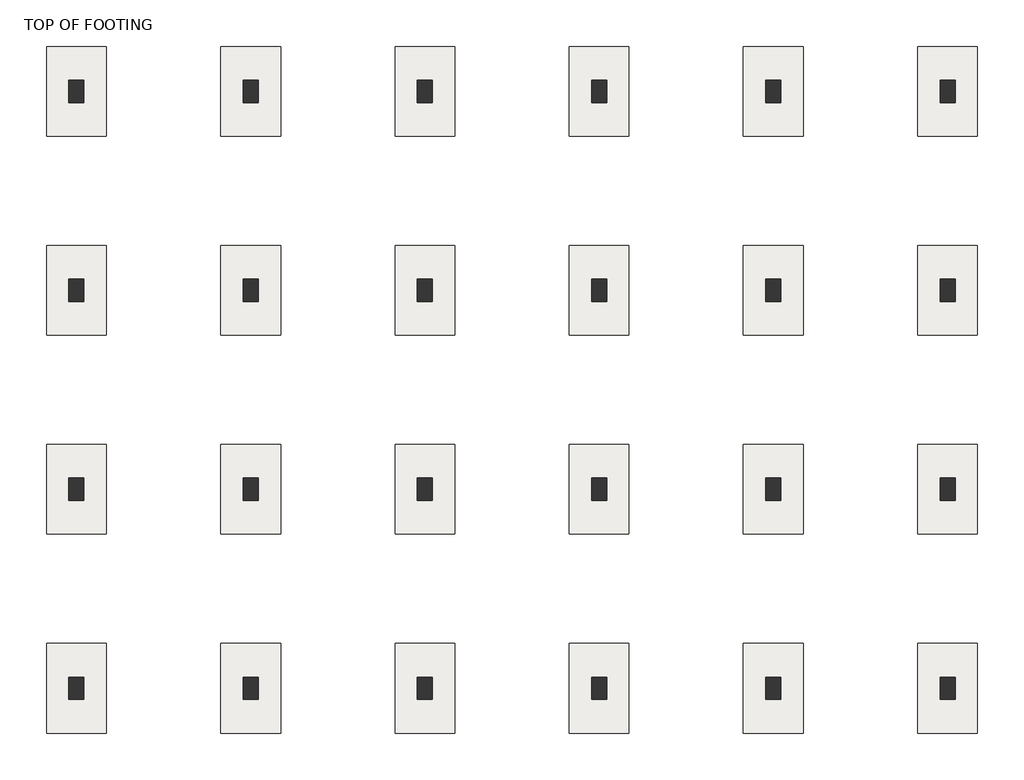
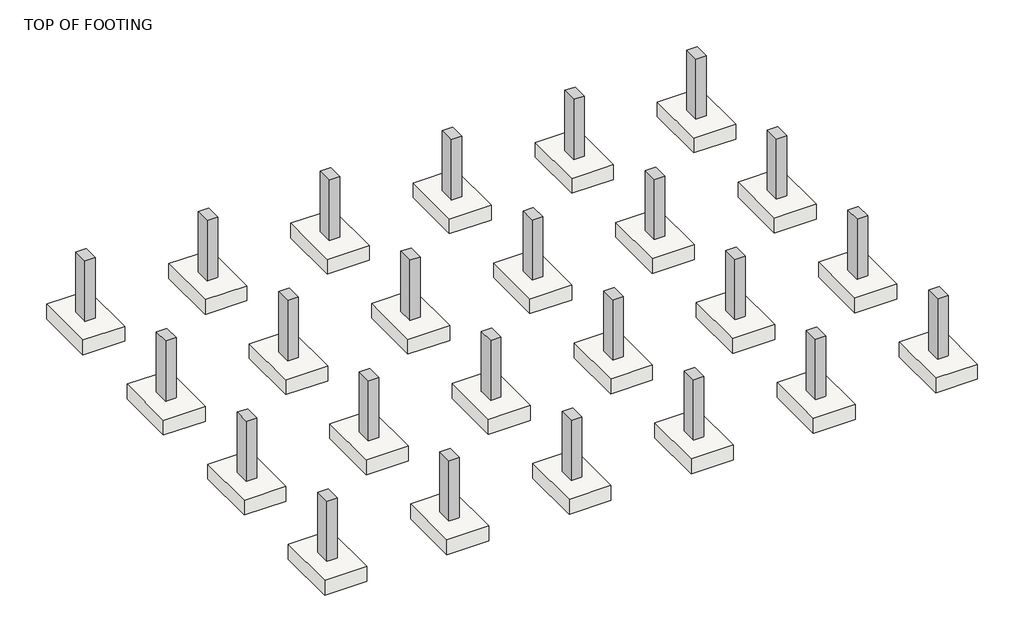
# One storey: 24 columns, 24 slabs.
"""IFC4 building model written with IfcOpenShell, lengths in millimetres."""

from ifc_helpers import new_model, si_unit, frame, origin, place, context, project, spatial, polyline, outline, extrude, transform, mapped, element, save
from components import m_footing_rectangular_1800_x_1200_x_450mm_16ba7ea5

model = new_model("IFC4")

# Units and contexts
model_context = context("Model", 3, world=origin())
ifc_project = project(units=[si_unit("LENGTHUNIT", "METRE", prefix="MILLI")], contexts=[model_context])

# Site, building, storey
site = spatial("IfcSite", under=ifc_project)
building = spatial("IfcBuilding", under=site)
storey = spatial("IfcBuildingStorey", under=building, Name="TOP OF FOOTING", Elevation=-1828.8)

# Columns
placement = place(None, origin())
element("IfcColumn", 1, ObjectType="M_Concrete-Rectangular-Column : 300 x 450mm", at=placement, inside=storey, context=model_context, shape_type="SweptSolid", body=[
    extrude(outline(polyline([(-8225.6838695, 17443.2036311), (-8225.6838695, 16993.2036311), (-8525.6838695, 16993.2036311), (-8525.6838695, 17443.2036311), (-8225.6838695, 17443.2036311)])), frame((0.0, 0.0, -1828.8), z_axis=(0.0, 0.0, 1.0), x_axis=(1.0, 0.0, 0.0)), (0.0, 0.0, 1.0), 1828.8),
])
element("IfcColumn", 2, ObjectType="M_Concrete-Rectangular-Column : 300 x 450mm", at=placement, inside=storey, context=model_context, shape_type="SweptSolid", body=[
    extrude(outline(polyline([(-4725.6838695, 17443.2036311), (-4725.6838695, 16993.2036311), (-5025.6838695, 16993.2036311), (-5025.6838695, 17443.2036311), (-4725.6838695, 17443.2036311)])), frame((0.0, 0.0, -1828.8), z_axis=(0.0, 0.0, 1.0), x_axis=(1.0, 0.0, 0.0)), (0.0, 0.0, 1.0), 1828.8),
])
element("IfcColumn", 3, ObjectType="M_Concrete-Rectangular-Column : 300 x 450mm", at=placement, inside=storey, context=model_context, shape_type="SweptSolid", body=[
    extrude(outline(polyline([(-1225.6838695, 17443.2036311), (-1225.6838695, 16993.2036311), (-1525.6838695, 16993.2036311), (-1525.6838695, 17443.2036311), (-1225.6838695, 17443.2036311)])), frame((0.0, 0.0, -1828.8), z_axis=(0.0, 0.0, 1.0), x_axis=(1.0, 0.0, 0.0)), (0.0, 0.0, 1.0), 1828.8),
])
element("IfcColumn", 4, ObjectType="M_Concrete-Rectangular-Column : 300 x 450mm", at=placement, inside=storey, context=model_context, shape_type="SweptSolid", body=[
    extrude(outline(polyline([(2274.3161305, 17443.2036311), (2274.3161305, 16993.2036311), (1974.3161305, 16993.2036311), (1974.3161305, 17443.2036311), (2274.3161305, 17443.2036311)])), frame((0.0, 0.0, -1828.8), z_axis=(0.0, 0.0, 1.0), x_axis=(1.0, 0.0, 0.0)), (0.0, 0.0, 1.0), 1828.8),
])
element("IfcColumn", 5, ObjectType="M_Concrete-Rectangular-Column : 300 x 450mm", at=placement, inside=storey, context=model_context, shape_type="SweptSolid", body=[
    extrude(outline(polyline([(5774.3161305, 17443.2036311), (5774.3161305, 16993.2036311), (5474.3161305, 16993.2036311), (5474.3161305, 17443.2036311), (5774.3161305, 17443.2036311)])), frame((0.0, 0.0, -1828.8), z_axis=(0.0, 0.0, 1.0), x_axis=(1.0, 0.0, 0.0)), (0.0, 0.0, 1.0), 1828.8),
])
element("IfcColumn", 6, ObjectType="M_Concrete-Rectangular-Column : 300 x 450mm", at=placement, inside=storey, context=model_context, shape_type="SweptSolid", body=[
    extrude(outline(polyline([(9274.3161305, 17443.2036311), (9274.3161305, 16993.2036311), (8974.3161305, 16993.2036311), (8974.3161305, 17443.2036311), (9274.3161305, 17443.2036311)])), frame((0.0, 0.0, -1828.8), z_axis=(0.0, 0.0, 1.0), x_axis=(1.0, 0.0, 0.0)), (0.0, 0.0, 1.0), 1828.8),
])
element("IfcColumn", 7, ObjectType="M_Concrete-Rectangular-Column : 300 x 450mm", at=placement, inside=storey, context=model_context, shape_type="SweptSolid", body=[
    extrude(outline(polyline([(9274.3161305, 13443.2036311), (9274.3161305, 12993.2036311), (8974.3161305, 12993.2036311), (8974.3161305, 13443.2036311), (9274.3161305, 13443.2036311)])), frame((0.0, 0.0, -1828.8), z_axis=(0.0, 0.0, 1.0), x_axis=(1.0, 0.0, 0.0)), (0.0, 0.0, 1.0), 1828.8),
])
element("IfcColumn", 8, ObjectType="M_Concrete-Rectangular-Column : 300 x 450mm", at=placement, inside=storey, context=model_context, shape_type="SweptSolid", body=[
    extrude(outline(polyline([(5774.3161305, 13443.2036311), (5774.3161305, 12993.2036311), (5474.3161305, 12993.2036311), (5474.3161305, 13443.2036311), (5774.3161305, 13443.2036311)])), frame((0.0, 0.0, -1828.8), z_axis=(0.0, 0.0, 1.0), x_axis=(1.0, 0.0, 0.0)), (0.0, 0.0, 1.0), 1828.8),
])
element("IfcColumn", 9, ObjectType="M_Concrete-Rectangular-Column : 300 x 450mm", at=placement, inside=storey, context=model_context, shape_type="SweptSolid", body=[
    extrude(outline(polyline([(2274.3161305, 13443.2036311), (2274.3161305, 12993.2036311), (1974.3161305, 12993.2036311), (1974.3161305, 13443.2036311), (2274.3161305, 13443.2036311)])), frame((0.0, 0.0, -1828.8), z_axis=(0.0, 0.0, 1.0), x_axis=(1.0, 0.0, 0.0)), (0.0, 0.0, 1.0), 1828.8),
])
element("IfcColumn", 10, ObjectType="M_Concrete-Rectangular-Column : 300 x 450mm", at=placement, inside=storey, context=model_context, shape_type="SweptSolid", body=[
    extrude(outline(polyline([(-1225.6838695, 13443.2036311), (-1225.6838695, 12993.2036311), (-1525.6838695, 12993.2036311), (-1525.6838695, 13443.2036311), (-1225.6838695, 13443.2036311)])), frame((0.0, 0.0, -1828.8), z_axis=(0.0, 0.0, 1.0), x_axis=(1.0, 0.0, 0.0)), (0.0, 0.0, 1.0), 1828.8),
])
element("IfcColumn", 11, ObjectType="M_Concrete-Rectangular-Column : 300 x 450mm", at=placement, inside=storey, context=model_context, shape_type="SweptSolid", body=[
    extrude(outline(polyline([(-4725.6838695, 13443.2036311), (-4725.6838695, 12993.2036311), (-5025.6838695, 12993.2036311), (-5025.6838695, 13443.2036311), (-4725.6838695, 13443.2036311)])), frame((0.0, 0.0, -1828.8), z_axis=(0.0, 0.0, 1.0), x_axis=(1.0, 0.0, 0.0)), (0.0, 0.0, 1.0), 1828.8),
])
element("IfcColumn", 12, ObjectType="M_Concrete-Rectangular-Column : 300 x 450mm", at=placement, inside=storey, context=model_context, shape_type="SweptSolid", body=[
    extrude(outline(polyline([(-8225.6838695, 13443.2036311), (-8225.6838695, 12993.2036311), (-8525.6838695, 12993.2036311), (-8525.6838695, 13443.2036311), (-8225.6838695, 13443.2036311)])), frame((0.0, 0.0, -1828.8), z_axis=(0.0, 0.0, 1.0), x_axis=(1.0, 0.0, 0.0)), (0.0, 0.0, 1.0), 1828.8),
])
element("IfcColumn", 13, ObjectType="M_Concrete-Rectangular-Column : 300 x 450mm", at=placement, inside=storey, context=model_context, shape_type="SweptSolid", body=[
    extrude(outline(polyline([(-8225.6838695, 9443.2036311), (-8225.6838695, 8993.2036311), (-8525.6838695, 8993.2036311), (-8525.6838695, 9443.2036311), (-8225.6838695, 9443.2036311)])), frame((0.0, 0.0, -1828.8), z_axis=(0.0, 0.0, 1.0), x_axis=(1.0, 0.0, 0.0)), (0.0, 0.0, 1.0), 1828.8),
])
element("IfcColumn", 14, ObjectType="M_Concrete-Rectangular-Column : 300 x 450mm", at=placement, inside=storey, context=model_context, shape_type="SweptSolid", body=[
    extrude(outline(polyline([(-4725.6838695, 9443.2036311), (-4725.6838695, 8993.2036311), (-5025.6838695, 8993.2036311), (-5025.6838695, 9443.2036311), (-4725.6838695, 9443.2036311)])), frame((0.0, 0.0, -1828.8), z_axis=(0.0, 0.0, 1.0), x_axis=(1.0, 0.0, 0.0)), (0.0, 0.0, 1.0), 1828.8),
])
element("IfcColumn", 15, ObjectType="M_Concrete-Rectangular-Column : 300 x 450mm", at=placement, inside=storey, context=model_context, shape_type="SweptSolid", body=[
    extrude(outline(polyline([(-1225.6838695, 9443.2036311), (-1225.6838695, 8993.2036311), (-1525.6838695, 8993.2036311), (-1525.6838695, 9443.2036311), (-1225.6838695, 9443.2036311)])), frame((0.0, 0.0, -1828.8), z_axis=(0.0, 0.0, 1.0), x_axis=(1.0, 0.0, 0.0)), (0.0, 0.0, 1.0), 1828.8),
])
element("IfcColumn", 16, ObjectType="M_Concrete-Rectangular-Column : 300 x 450mm", at=placement, inside=storey, context=model_context, shape_type="SweptSolid", body=[
    extrude(outline(polyline([(2274.3161305, 9443.2036311), (2274.3161305, 8993.2036311), (1974.3161305, 8993.2036311), (1974.3161305, 9443.2036311), (2274.3161305, 9443.2036311)])), frame((0.0, 0.0, -1828.8), z_axis=(0.0, 0.0, 1.0), x_axis=(1.0, 0.0, 0.0)), (0.0, 0.0, 1.0), 1828.8),
])
element("IfcColumn", 17, ObjectType="M_Concrete-Rectangular-Column : 300 x 450mm", at=placement, inside=storey, context=model_context, shape_type="SweptSolid", body=[
    extrude(outline(polyline([(5774.3161305, 9443.2036311), (5774.3161305, 8993.2036311), (5474.3161305, 8993.2036311), (5474.3161305, 9443.2036311), (5774.3161305, 9443.2036311)])), frame((0.0, 0.0, -1828.8), z_axis=(0.0, 0.0, 1.0), x_axis=(1.0, 0.0, 0.0)), (0.0, 0.0, 1.0), 1828.8),
])
element("IfcColumn", 18, ObjectType="M_Concrete-Rectangular-Column : 300 x 450mm", at=placement, inside=storey, context=model_context, shape_type="SweptSolid", body=[
    extrude(outline(polyline([(9274.3161305, 9443.2036311), (9274.3161305, 8993.2036311), (8974.3161305, 8993.2036311), (8974.3161305, 9443.2036311), (9274.3161305, 9443.2036311)])), frame((0.0, 0.0, -1828.8), z_axis=(0.0, 0.0, 1.0), x_axis=(1.0, 0.0, 0.0)), (0.0, 0.0, 1.0), 1828.8),
])
element("IfcColumn", 19, ObjectType="M_Concrete-Rectangular-Column : 300 x 450mm", at=placement, inside=storey, context=model_context, shape_type="SweptSolid", body=[
    extrude(outline(polyline([(9274.3161305, 5443.2036311), (9274.3161305, 4993.2036311), (8974.3161305, 4993.2036311), (8974.3161305, 5443.2036311), (9274.3161305, 5443.2036311)])), frame((0.0, 0.0, -1828.8), z_axis=(0.0, 0.0, 1.0), x_axis=(1.0, 0.0, 0.0)), (0.0, 0.0, 1.0), 1828.8),
])
element("IfcColumn", 20, ObjectType="M_Concrete-Rectangular-Column : 300 x 450mm", at=placement, inside=storey, context=model_context, shape_type="SweptSolid", body=[
    extrude(outline(polyline([(5774.3161305, 5443.2036311), (5774.3161305, 4993.2036311), (5474.3161305, 4993.2036311), (5474.3161305, 5443.2036311), (5774.3161305, 5443.2036311)])), frame((0.0, 0.0, -1828.8), z_axis=(0.0, 0.0, 1.0), x_axis=(1.0, 0.0, 0.0)), (0.0, 0.0, 1.0), 1828.8),
])
element("IfcColumn", 21, ObjectType="M_Concrete-Rectangular-Column : 300 x 450mm", at=placement, inside=storey, context=model_context, shape_type="SweptSolid", body=[
    extrude(outline(polyline([(2274.3161305, 5443.2036311), (2274.3161305, 4993.2036311), (1974.3161305, 4993.2036311), (1974.3161305, 5443.2036311), (2274.3161305, 5443.2036311)])), frame((0.0, 0.0, -1828.8), z_axis=(0.0, 0.0, 1.0), x_axis=(1.0, 0.0, 0.0)), (0.0, 0.0, 1.0), 1828.8),
])
element("IfcColumn", 22, ObjectType="M_Concrete-Rectangular-Column : 300 x 450mm", at=placement, inside=storey, context=model_context, shape_type="SweptSolid", body=[
    extrude(outline(polyline([(-1225.6838695, 5443.2036311), (-1225.6838695, 4993.2036311), (-1525.6838695, 4993.2036311), (-1525.6838695, 5443.2036311), (-1225.6838695, 5443.2036311)])), frame((0.0, 0.0, -1828.8), z_axis=(0.0, 0.0, 1.0), x_axis=(1.0, 0.0, 0.0)), (0.0, 0.0, 1.0), 1828.8),
])
element("IfcColumn", 23, ObjectType="M_Concrete-Rectangular-Column : 300 x 450mm", at=placement, inside=storey, context=model_context, shape_type="SweptSolid", body=[
    extrude(outline(polyline([(-4725.6838695, 5443.2036311), (-4725.6838695, 4993.2036311), (-5025.6838695, 4993.2036311), (-5025.6838695, 5443.2036311), (-4725.6838695, 5443.2036311)])), frame((0.0, 0.0, -1828.8), z_axis=(0.0, 0.0, 1.0), x_axis=(1.0, 0.0, 0.0)), (0.0, 0.0, 1.0), 1828.8),
])
element("IfcColumn", 24, ObjectType="M_Concrete-Rectangular-Column : 300 x 450mm", at=placement, inside=storey, context=model_context, shape_type="SweptSolid", body=[
    extrude(outline(polyline([(-8225.6838695, 5443.2036311), (-8225.6838695, 4993.2036311), (-8525.6838695, 4993.2036311), (-8525.6838695, 5443.2036311), (-8225.6838695, 5443.2036311)])), frame((0.0, 0.0, -1828.8), z_axis=(0.0, 0.0, 1.0), x_axis=(1.0, 0.0, 0.0)), (0.0, 0.0, 1.0), 1828.8),
])

# Slabs
m_footing_rectangular_1800_x_1200_x_450mm_shape = m_footing_rectangular_1800_x_1200_x_450mm_16ba7ea5(model_context)
element("IfcSlab", 25, ObjectType="M_Footing-Rectangular : 1800 x 1200 x 450mm", at=placement, inside=storey, context=model_context, shape_type="MappedRepresentation", body=[
    mapped(m_footing_rectangular_1800_x_1200_x_450mm_shape, transform((-8375.6838695, 17218.2036311, -1828.8), x_axis=(1.0, 0.0, 0.0), y_axis=(0.0, 1.0, 0.0), z_axis=(0.0, 0.0, 1.0))),
])
element("IfcSlab", 26, ObjectType="M_Footing-Rectangular : 1800 x 1200 x 450mm", at=placement, inside=storey, context=model_context, shape_type="MappedRepresentation", body=[
    mapped(m_footing_rectangular_1800_x_1200_x_450mm_shape, transform((-4875.6838695, 17218.2036311, -1828.8), x_axis=(1.0, 0.0, 0.0), y_axis=(0.0, 1.0, 0.0), z_axis=(0.0, 0.0, 1.0))),
])
element("IfcSlab", 27, ObjectType="M_Footing-Rectangular : 1800 x 1200 x 450mm", at=placement, inside=storey, context=model_context, shape_type="MappedRepresentation", body=[
    mapped(m_footing_rectangular_1800_x_1200_x_450mm_shape, transform((-1375.6838695, 17218.2036311, -1828.8), x_axis=(1.0, 0.0, 0.0), y_axis=(0.0, 1.0, 0.0), z_axis=(0.0, 0.0, 1.0))),
])
element("IfcSlab", 28, ObjectType="M_Footing-Rectangular : 1800 x 1200 x 450mm", at=placement, inside=storey, context=model_context, shape_type="MappedRepresentation", body=[
    mapped(m_footing_rectangular_1800_x_1200_x_450mm_shape, transform((2124.3161305, 17218.2036311, -1828.8), x_axis=(1.0, 0.0, 0.0), y_axis=(0.0, 1.0, 0.0), z_axis=(0.0, 0.0, 1.0))),
])
element("IfcSlab", 29, ObjectType="M_Footing-Rectangular : 1800 x 1200 x 450mm", at=placement, inside=storey, context=model_context, shape_type="MappedRepresentation", body=[
    mapped(m_footing_rectangular_1800_x_1200_x_450mm_shape, transform((5624.3161305, 17218.2036311, -1828.8), x_axis=(1.0, 0.0, 0.0), y_axis=(0.0, 1.0, 0.0), z_axis=(0.0, 0.0, 1.0))),
])
element("IfcSlab", 30, ObjectType="M_Footing-Rectangular : 1800 x 1200 x 450mm", at=placement, inside=storey, context=model_context, shape_type="MappedRepresentation", body=[
    mapped(m_footing_rectangular_1800_x_1200_x_450mm_shape, transform((9124.3161305, 17218.2036311, -1828.8), x_axis=(1.0, 0.0, 0.0), y_axis=(0.0, 1.0, 0.0), z_axis=(0.0, 0.0, 1.0))),
])
element("IfcSlab", 31, ObjectType="M_Footing-Rectangular : 1800 x 1200 x 450mm", at=placement, inside=storey, context=model_context, shape_type="MappedRepresentation", body=[
    mapped(m_footing_rectangular_1800_x_1200_x_450mm_shape, transform((9124.3161305, 13218.2036311, -1828.8), x_axis=(1.0, 0.0, 0.0), y_axis=(0.0, 1.0, 0.0), z_axis=(0.0, 0.0, 1.0))),
])
element("IfcSlab", 32, ObjectType="M_Footing-Rectangular : 1800 x 1200 x 450mm", at=placement, inside=storey, context=model_context, shape_type="MappedRepresentation", body=[
    mapped(m_footing_rectangular_1800_x_1200_x_450mm_shape, transform((5624.3161305, 13218.2036311, -1828.8), x_axis=(1.0, 0.0, 0.0), y_axis=(0.0, 1.0, 0.0), z_axis=(0.0, 0.0, 1.0))),
])
element("IfcSlab", 33, ObjectType="M_Footing-Rectangular : 1800 x 1200 x 450mm", at=placement, inside=storey, context=model_context, shape_type="MappedRepresentation", body=[
    mapped(m_footing_rectangular_1800_x_1200_x_450mm_shape, transform((2124.3161305, 13218.2036311, -1828.8), x_axis=(1.0, 0.0, 0.0), y_axis=(0.0, 1.0, 0.0), z_axis=(0.0, 0.0, 1.0))),
])
element("IfcSlab", 34, ObjectType="M_Footing-Rectangular : 1800 x 1200 x 450mm", at=placement, inside=storey, context=model_context, shape_type="MappedRepresentation", body=[
    mapped(m_footing_rectangular_1800_x_1200_x_450mm_shape, transform((-1375.6838695, 13218.2036311, -1828.8), x_axis=(1.0, 0.0, 0.0), y_axis=(0.0, 1.0, 0.0), z_axis=(0.0, 0.0, 1.0))),
])
element("IfcSlab", 35, ObjectType="M_Footing-Rectangular : 1800 x 1200 x 450mm", at=placement, inside=storey, context=model_context, shape_type="MappedRepresentation", body=[
    mapped(m_footing_rectangular_1800_x_1200_x_450mm_shape, transform((-4875.6838695, 13218.2036311, -1828.8), x_axis=(1.0, 0.0, 0.0), y_axis=(0.0, 1.0, 0.0), z_axis=(0.0, 0.0, 1.0))),
])
element("IfcSlab", 36, ObjectType="M_Footing-Rectangular : 1800 x 1200 x 450mm", at=placement, inside=storey, context=model_context, shape_type="MappedRepresentation", body=[
    mapped(m_footing_rectangular_1800_x_1200_x_450mm_shape, transform((-8375.6838695, 13218.2036311, -1828.8), x_axis=(1.0, 0.0, 0.0), y_axis=(0.0, 1.0, 0.0), z_axis=(0.0, 0.0, 1.0))),
])
element("IfcSlab", 37, ObjectType="M_Footing-Rectangular : 1800 x 1200 x 450mm", at=placement, inside=storey, context=model_context, shape_type="MappedRepresentation", body=[
    mapped(m_footing_rectangular_1800_x_1200_x_450mm_shape, transform((-8375.6838695, 9218.2036311, -1828.8), x_axis=(1.0, 0.0, 0.0), y_axis=(0.0, 1.0, 0.0), z_axis=(0.0, 0.0, 1.0))),
])
element("IfcSlab", 38, ObjectType="M_Footing-Rectangular : 1800 x 1200 x 450mm", at=placement, inside=storey, context=model_context, shape_type="MappedRepresentation", body=[
    mapped(m_footing_rectangular_1800_x_1200_x_450mm_shape, transform((-4875.6838695, 9218.2036311, -1828.8), x_axis=(1.0, 0.0, 0.0), y_axis=(0.0, 1.0, 0.0), z_axis=(0.0, 0.0, 1.0))),
])
element("IfcSlab", 39, ObjectType="M_Footing-Rectangular : 1800 x 1200 x 450mm", at=placement, inside=storey, context=model_context, shape_type="MappedRepresentation", body=[
    mapped(m_footing_rectangular_1800_x_1200_x_450mm_shape, transform((-1375.6838695, 9218.2036311, -1828.8), x_axis=(1.0, 0.0, 0.0), y_axis=(0.0, 1.0, 0.0), z_axis=(0.0, 0.0, 1.0))),
])
element("IfcSlab", 40, ObjectType="M_Footing-Rectangular : 1800 x 1200 x 450mm", at=placement, inside=storey, context=model_context, shape_type="MappedRepresentation", body=[
    mapped(m_footing_rectangular_1800_x_1200_x_450mm_shape, transform((2124.3161305, 9218.2036311, -1828.8), x_axis=(1.0, 0.0, 0.0), y_axis=(0.0, 1.0, 0.0), z_axis=(0.0, 0.0, 1.0))),
])
element("IfcSlab", 41, ObjectType="M_Footing-Rectangular : 1800 x 1200 x 450mm", at=placement, inside=storey, context=model_context, shape_type="MappedRepresentation", body=[
    mapped(m_footing_rectangular_1800_x_1200_x_450mm_shape, transform((5624.3161305, 9218.2036311, -1828.8), x_axis=(1.0, 0.0, 0.0), y_axis=(0.0, 1.0, 0.0), z_axis=(0.0, 0.0, 1.0))),
])
element("IfcSlab", 42, ObjectType="M_Footing-Rectangular : 1800 x 1200 x 450mm", at=placement, inside=storey, context=model_context, shape_type="MappedRepresentation", body=[
    mapped(m_footing_rectangular_1800_x_1200_x_450mm_shape, transform((9124.3161305, 9218.2036311, -1828.8), x_axis=(1.0, 0.0, 0.0), y_axis=(0.0, 1.0, 0.0), z_axis=(0.0, 0.0, 1.0))),
])
element("IfcSlab", 43, ObjectType="M_Footing-Rectangular : 1800 x 1200 x 450mm", at=placement, inside=storey, context=model_context, shape_type="MappedRepresentation", body=[
    mapped(m_footing_rectangular_1800_x_1200_x_450mm_shape, transform((9124.3161305, 5218.2036311, -1828.8), x_axis=(1.0, 0.0, 0.0), y_axis=(0.0, 1.0, 0.0), z_axis=(0.0, 0.0, 1.0))),
])
element("IfcSlab", 44, ObjectType="M_Footing-Rectangular : 1800 x 1200 x 450mm", at=placement, inside=storey, context=model_context, shape_type="MappedRepresentation", body=[
    mapped(m_footing_rectangular_1800_x_1200_x_450mm_shape, transform((5624.3161305, 5218.2036311, -1828.8), x_axis=(1.0, 0.0, 0.0), y_axis=(0.0, 1.0, 0.0), z_axis=(0.0, 0.0, 1.0))),
])
element("IfcSlab", 45, ObjectType="M_Footing-Rectangular : 1800 x 1200 x 450mm", at=placement, inside=storey, context=model_context, shape_type="MappedRepresentation", body=[
    mapped(m_footing_rectangular_1800_x_1200_x_450mm_shape, transform((2124.3161305, 5218.2036311, -1828.8), x_axis=(1.0, 0.0, 0.0), y_axis=(0.0, 1.0, 0.0), z_axis=(0.0, 0.0, 1.0))),
])
element("IfcSlab", 46, ObjectType="M_Footing-Rectangular : 1800 x 1200 x 450mm", at=placement, inside=storey, context=model_context, shape_type="MappedRepresentation", body=[
    mapped(m_footing_rectangular_1800_x_1200_x_450mm_shape, transform((-1375.6838695, 5218.2036311, -1828.8), x_axis=(1.0, 0.0, 0.0), y_axis=(0.0, 1.0, 0.0), z_axis=(0.0, 0.0, 1.0))),
])
element("IfcSlab", 47, ObjectType="M_Footing-Rectangular : 1800 x 1200 x 450mm", at=placement, inside=storey, context=model_context, shape_type="MappedRepresentation", body=[
    mapped(m_footing_rectangular_1800_x_1200_x_450mm_shape, transform((-4875.6838695, 5218.2036311, -1828.8), x_axis=(1.0, 0.0, 0.0), y_axis=(0.0, 1.0, 0.0), z_axis=(0.0, 0.0, 1.0))),
])
element("IfcSlab", 48, ObjectType="M_Footing-Rectangular : 1800 x 1200 x 450mm", at=placement, inside=storey, context=model_context, shape_type="MappedRepresentation", body=[
    mapped(m_footing_rectangular_1800_x_1200_x_450mm_shape, transform((-8375.6838695, 5218.2036311, -1828.8), x_axis=(1.0, 0.0, 0.0), y_axis=(0.0, 1.0, 0.0), z_axis=(0.0, 0.0, 1.0))),
])

save(model, "model.ifc")

# Revit data of these elements
# Grids (mm)
#   "4": line (2124.316, 19418.46) -> (2124.316, -11457.83)
#   "D": line (10909.931, 5218.204) -> (-10310.934, 5218.204)
#   "1": line (-8375.684, 19418.46) -> (-8375.684, -11457.83)
#   "2": line (-4875.684, 19418.46) -> (-4875.684, -11457.83)
#   "3": line (-1375.684, 19418.46) -> (-1375.684, -11457.83)
#   "5": line (5624.316, 19418.46) -> (5624.316, -11457.83)
#   "6": line (9124.316, 19418.46) -> (9124.316, -11457.83)
#   "A": line (10909.931, 17218.204) -> (-10310.934, 17218.204)
#   "B": line (10909.931, 13218.204) -> (-10310.934, 13218.204)
#   "C": line (10909.931, 9218.204) -> (-10310.934, 9218.204)
# Type "M_Concrete-Rectangular-Column : 300 x 450mm"
#   b = 300 mm
#   h = 450 mm
#   Structural Material [instance default] = Concrete, Cast-in-Place gray
# Type "M_Footing-Rectangular : 1800 x 1200 x 450mm"
#   Width = 1200 mm
#   Length = 1800 mm
#   Foundation Thickness = 450 mm
#   Structural Material [instance default] = Concrete, Cast-in-Place gray
#   Assembly Code = ""
# Elements 1, 2, 3, 4, 5, 6, 7, 8, 9, 10, 11, 12, 13, 14, 15, 16, 17, 18, 19, 20, 21, 22, 23, 24 (IfcColumn, "M_Concrete-Rectangular-Column : 300 x 450mm")
#   Structural Material = Concrete, Cast-in-Place gray
#   Phase Created = New Construction
#   Materials on its faces: "Concrete, Cast-in-Place gray"
# Elements 25, 26, 27, 28, 29, 30, 31, 32, 33, 34, 35, 36, 37, 38, 39, 40, 41, 42, 43, 44, 45, 46, 47, 48 (IfcSlab, "M_Footing-Rectangular : 1800 x 1200 x 450mm")
#   Structural Material = Concrete, Cast-in-Place gray
#   Phase Created = New Construction
#   Materials on its faces: "Concrete, Cast-in-Place gray"
# Materials
#   "Concrete, Cast-in-Place gray": class "Concrete", colour RGB 192 192 192, transparency 0, Description = "Cast-in-place concrete", Cost = 0
